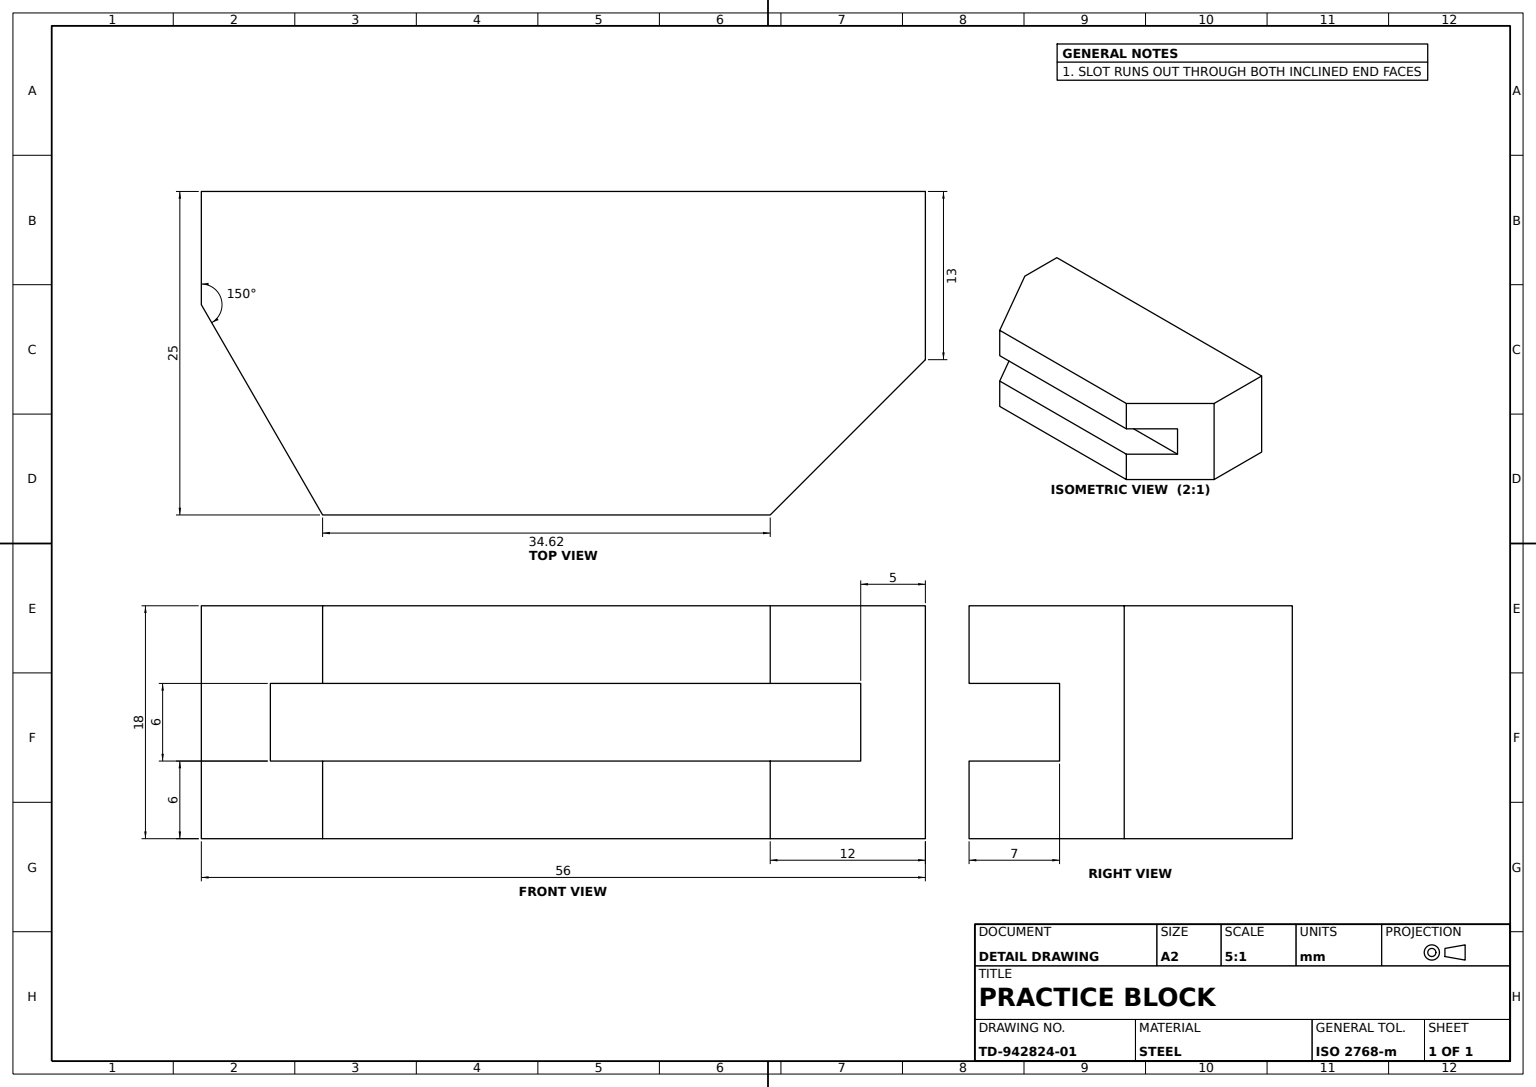
SolidWorks part; units mm, degrees
material "Plain Carbon Steel"
ref_plane "Front Plane" through (0, 0, 0) normal (0, 0, 1) x (1, 0, 0)
ref_plane "Top Plane" through (0, 0, 0) normal (0, 1, 0) x (1, 0, 0)
ref_plane "Right Plane" through (0, 0, 0) normal (1, 0, 0) x (0, 0, -1)
sketch "Base Profile Sketch" plane through (0, 0, 0) normal (0, 0, 1) x (1, 0, 0)
  line L1 (-28, -9) -> (28, -9)
  line L2 (-28, -9) -> (-28, 9)
  line L3 (-28, 9) -> (28, 9)
  line L4 (28, -9) -> (28, 9)
  line L5 (-28, -9) -> (28, 9) construction
  line L6 (-28, 9) -> (28, -9) construction
  point P0 (0, 0)
  dimension "D1" = 56
  dimension "D2" = 18
extrude "Base Block" add sketch "Base Profile Sketch" along normal blind 25
sketch "Corner Cut Sketch" plane through (0, -9, 0) normal (0, -1, 0) x (1, 0, 0)
  line L0 (28, 13) -> (16, 25)
  line L2 (-28, 25) -> (28, 25) construction
  line L3 (-28, 0) -> (28, 0) construction
  line L5 (-28, 25) -> (-28, 0) construction
  line L6 (-28, 13) -> (-28, 8.7531)
  line L7 (-28, 25) -> (-18.6198, 25)
  line L8 (-28, 8.7531) -> (-28, 25) construction
  line L9 (-28, 8.7531) -> (-18.6198, 25)
  line L10 (16, 25) -> (28, 25)
  line L11 (-28, 13) -> (-28, 25)
  line L12 (28, 13) -> (28, 25)
  dimension "D1" = 13
  dimension "D2" = 56
  dimension "D3" = 13
  dimension "D4" = 150
  dimension "D5" = 12
  dimension "D6" = 34.6198
extrude "Angled Corner Cuts" cut sketch "Corner Cut Sketch" against normal through all
sketch "Slot Sketch" plane through (0, 0, 25) normal (0, 0, 1) x (1, 0, 0)
  line L1 (-23.5, -3) -> (23.5, -3)
  line L2 (-23.5, -3) -> (-23.5, 3)
  line L3 (-23.5, 3) -> (23.5, 3)
  line L4 (23.5, -3) -> (23.5, 3)
  line L5 (-23.5, -3) -> (23.5, 3) construction
  line L6 (-23.5, 3) -> (23.5, -3) construction
  point P0 (0, 0)
  dimension "D1" = 47
  dimension "D2" = 6
extrude "Slot 47x6" cut sketch "Slot Sketch" against normal blind 7
